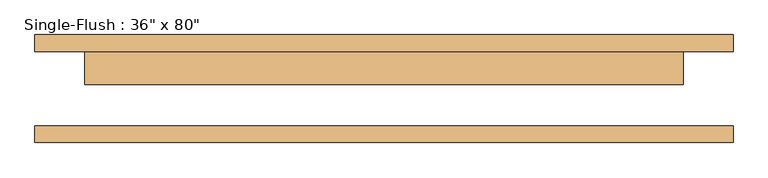
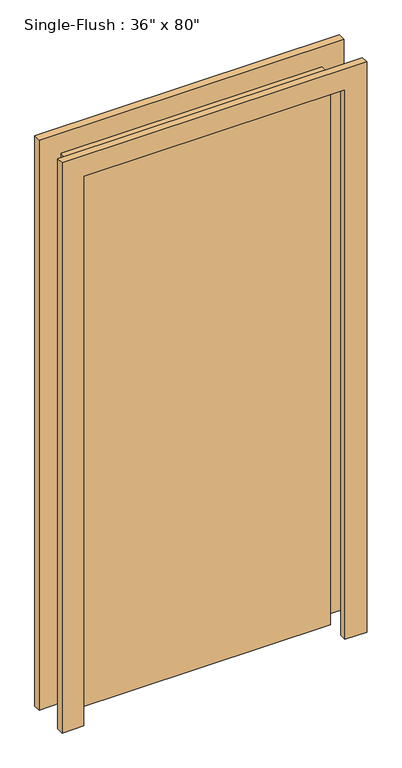
"""IFC4 building model written with IfcOpenShell, lengths in millimetres: door geometry."""

from ifc_helpers import new_model, si_unit, frame, origin, origin_with_axes, place, context, project, spatial, polyline, outline, extrude, source, transform, mapped, element, save


def door_17d80c48(model_context):
    return source(origin(), model_context, "Body", "SweptSolid", [
        extrude(outline(polyline([(2108.2, -533.4), (0.0, -533.4), (0.0, -457.2), (2032.0, -457.2), (2032.0, 457.2), (0.0, 457.2), (0.0, 533.4), (2108.2, 533.4), (2108.2, -533.4)])), frame((0.0, 57.15, 0.0), z_axis=(0.0, 1.0, 0.0), x_axis=(0.0, 0.0, 1.0)), (0.0, 0.0, 1.0), 25.4),
        extrude(outline(polyline([(2108.2, 533.4), (2108.2, -533.4), (0.0, -533.4), (0.0, -457.2), (2032.0, -457.2), (2032.0, 457.2), (0.0, 457.2), (0.0, 533.4), (2108.2, 533.4)])), frame((0.0, -82.55, 0.0), z_axis=(0.0, 1.0, 0.0), x_axis=(0.0, 0.0, 1.0)), (0.0, 0.0, 1.0), 25.4),
        extrude(outline(polyline([(457.2, 6.35), (-457.2, 6.35), (-457.2, 57.15), (457.2, 57.15), (457.2, 6.35)])), origin_with_axes(), (0.0, 0.0, 1.0), 2032.0),
    ])


if __name__ == "__main__":
    model = new_model("IFC4")
    model_context = context("Model", 3, world=origin())
    ifc_project = project(units=[si_unit("LENGTHUNIT", "METRE", prefix="MILLI")], contexts=[model_context])
    site = spatial("IfcSite", under=ifc_project)
    building = spatial("IfcBuilding", under=site)
    placement = place(None, origin())
    door_shape = door_17d80c48(model_context)
    element("IfcDoor", 1, ObjectType="Single-Flush : 36\" x 80\"", at=placement, inside=building, context=model_context, shape_type="MappedRepresentation", body=[
        mapped(door_shape, transform((0.0, 0.0, 0.0), x_axis=(1.0, 0.0, 0.0), y_axis=(0.0, 1.0, 0.0), z_axis=(0.0, 0.0, 1.0))),
    ])
    save(model, "model.ifc")

# Revit data of these elements
# Type "Single-Flush : 36\" x 80\""
#   Type Mark = "6"
#   Construction Type Id = "MDOOR"
#   Assembly Code = "C1020"
#   Analytic Construction = "Metal"
#   Thickness = 0' - 2"
#   Heat Transfer Coefficient (U) = 0.651978 BTU/(h·ft²·°F)
#   Height = 6' - 8"
#   Trim Projection Ext = 0' - 1"
#   Trim Projection Int = 0' - 1"
#   Trim Width = 0' - 3"
#   Width = 3' - 0"
#   Define Thermal Properties by = 1
#   Define Thermal Properties by = 1
#   Door Material = Door - Panel
#   Frame Material = Door - Frame
#   Visual Light Transmittance = 0
#   Solar Heat Gain Coefficient = 0
#   Function = (empty or 0)
#   Wall Closure = (empty or 0)
# Element 1 (IfcDoor, "Single-Flush : 36\" x 80\"")
#   Materials on its faces: "Door - Frame", "Door - Panel"
# Materials
#   "Door - Panel": class "Wood", colour RGB 210 159 95, transparency 0, Cost = 0
#   "Door - Frame": colour RGB 118 70 51, transparency 0, Cost = 0
